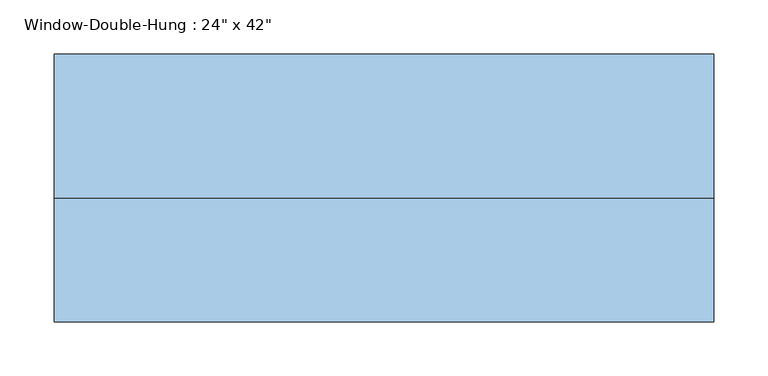
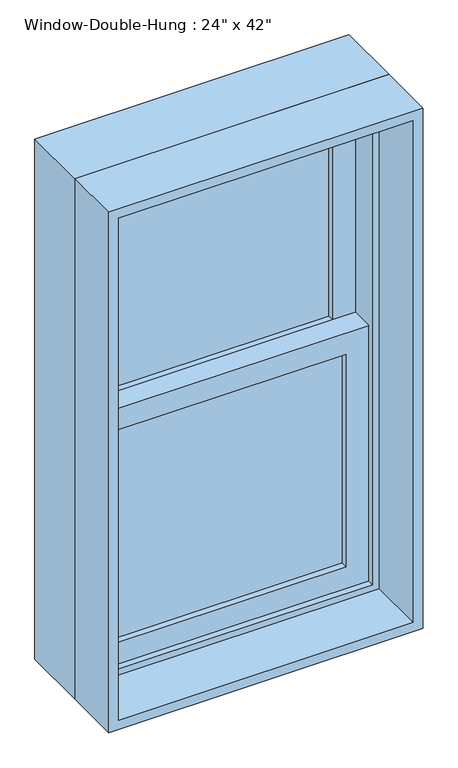
"""IFC4 building model written with IfcOpenShell, lengths in millimetres: window geometry."""

from ifc_helpers import new_model, si_unit, frame, origin, place, context, project, spatial, polyline, outline, extrude, source, transform, mapped, element, save


def window_d92165b9(model_context):
    return source(origin(), model_context, "Body", "SweptSolid", [
        extrude(outline(polyline([(228.6, 44.45), (228.6, 38.1), (-228.6, 38.1), (-228.6, 44.45), (228.6, 44.45)])), frame((0.0, 0.0, 990.6), z_axis=(0.0, 0.0, 1.0), x_axis=(1.0, 0.0, 0.0)), (0.0, 0.0, 1.0), 434.975),
        extrude(outline(polyline([(-228.6, 31.75), (228.6, 31.75), (228.6, 25.4), (-228.6, 25.4), (-228.6, 31.75)])), frame((0.0, 0.0, 990.6), z_axis=(0.0, 0.0, 1.0), x_axis=(1.0, 0.0, 0.0)), (0.0, 0.0, 1.0), 434.975),
        extrude(outline(polyline([(228.6, 88.9), (228.6, 82.55), (-228.6, 82.55), (-228.6, 88.9), (228.6, 88.9)])), frame((0.0, 0.0, 1470.025), z_axis=(0.0, 0.0, 1.0), x_axis=(1.0, 0.0, 0.0)), (0.0, 0.0, 1.0), 434.975),
        extrude(outline(polyline([(-228.6, 76.2), (228.6, 76.2), (228.6, 69.85), (-228.6, 69.85), (-228.6, 76.2)])), frame((0.0, 0.0, 1470.025), z_axis=(0.0, 0.0, 1.0), x_axis=(1.0, 0.0, 0.0)), (0.0, 0.0, 1.0), 434.975),
        extrude(outline(polyline([(1470.025, -273.05), (946.15, -273.05), (946.15, 273.05), (1470.025, 273.05), (1470.025, -273.05)]), holes=[polyline([(1425.575, 228.6), (990.6, 228.6), (990.6, -228.6), (1425.575, -228.6), (1425.575, 228.6)])]), frame((0.0, 12.7, 0.0), z_axis=(0.0, 1.0, 0.0), x_axis=(0.0, 0.0, 1.0)), (0.0, 0.0, 1.0), 44.45),
        extrude(outline(polyline([(1949.45, -273.05), (1425.575, -273.05), (1425.575, 273.05), (1949.45, 273.05), (1949.45, -273.05)]), holes=[polyline([(1905.0, 228.6), (1470.025, 228.6), (1470.025, -228.6), (1905.0, -228.6), (1905.0, 228.6)])]), frame((0.0, 57.15, 0.0), z_axis=(0.0, 1.0, 0.0), x_axis=(0.0, 0.0, 1.0)), (0.0, 0.0, 1.0), 44.45),
        extrude(outline(polyline([(1981.2, -304.8), (914.4, -304.8), (914.4, 304.8), (1981.2, 304.8), (1981.2, -304.8)]), holes=[polyline([(1949.45, 273.05), (946.15, 273.05), (946.15, -273.05), (1949.45, -273.05), (1949.45, 273.05)])]), frame((0.0, 0.0, 0.0), z_axis=(0.0, 1.0, 0.0), x_axis=(0.0, 0.0, 1.0)), (0.0, 0.0, 1.0), 133.35),
        extrude(outline(polyline([(1981.2, 304.8), (1981.2, -304.8), (914.4, -304.8), (914.4, 304.8), (1981.2, 304.8)]), holes=[polyline([(1962.15, 285.75), (933.45, 285.75), (933.45, -285.75), (1962.15, -285.75), (1962.15, 285.75)])]), frame((0.0, -114.3, 0.0), z_axis=(0.0, 1.0, 0.0), x_axis=(0.0, 0.0, 1.0)), (0.0, 0.0, 1.0), 114.3),
    ])


if __name__ == "__main__":
    model = new_model("IFC4")
    model_context = context("Model", 3, world=origin())
    ifc_project = project(units=[si_unit("LENGTHUNIT", "METRE", prefix="MILLI")], contexts=[model_context])
    site = spatial("IfcSite", under=ifc_project)
    building = spatial("IfcBuilding", under=site)
    placement = place(None, origin())
    window_shape = window_d92165b9(model_context)
    element("IfcWindow", 1, ObjectType="Window-Double-Hung : 24\" x 42\"", at=placement, inside=building, context=model_context, shape_type="MappedRepresentation", body=[
        mapped(window_shape, transform((0.0, 0.0, 0.0), x_axis=(1.0, 0.0, 0.0), y_axis=(0.0, 1.0, 0.0), z_axis=(0.0, 0.0, 1.0))),
    ])
    save(model, "model.ifc")

# Revit data of these elements
# Type "Window-Double-Hung : 24\" x 42\""
#   Type Mark = "10"
#   Fire Rating = "0.5h"
#   Construction Type Id = "DG-DR"
#   Assembly Code = "B2020100"
#   Analytic Construction = "Double glazing - domestic"
#   Wall Thickness [instance default] = 0' - 6"
#   Window Inset [instance default] = 0' - 0"
#   Visual Light Transmittance = 0.81
#   Thermal Resistance (R) = 1.8146 (h·ft²·°F)/BTU
#   Solar Heat Gain Coefficient = 0.76
#   Muntin Width = 1' - 6"
#   Muntin Height = 1' - 5 1/8"
#   Interior Wall Closure [instance default] = 0' - 1 1/2"
#   Rough Width = 2' - 0 1/2"
#   Rough Height = 3' - 6 1/2"
#   Frame Extension [instance default] = 0' - 1 1/4"
#   Exterior Wall Closure [instance default] = 0' - 0 1/2"
#   Extension Jamb [instance default] = 0' - 1 1/2"
#   Heat Transfer Coefficient (U) = 0.5511 BTU/(h·ft²·°F)
#   Height = 3' - 6"
#   Width = 2' - 0"
#   Define Thermal Properties by = 1
#   Top Muntin Visibility = yes
#   Indicator Visibility [instance default] = yes
#   Extension Jamb Visibility [instance default] = yes
#   Interior Trim Visibility [instance default] = yes
#   Exterior Trim Visibility [instance default] = yes
#   Define Thermal Properties by = 1
#   Bottom Muntin Visibility = yes
#   Muntin Pattern = Muntin Pattern_2x2 : Muntin Pattern_2x2
#   Interior Trim Material = Wood - Stained
#   Interior Trim = Trim-Window-Interior-Flat : Picture Frame
#   Exterior Trim Material = Clad - White
#   Exterior Trim = Trim-Window-Exterior-Flat : with Sill
#   Glass Panel Material = Glass
#   Exterior Frame Material = Clad - White
#   Interior Frame Material = Wood - Stained
#   Wall Closure = (empty or 0)
# Element 1 (IfcWindow, "Window-Double-Hung : 24\" x 42\"")
#   Wall Thickness = 0' - 9"
#   Extension Jamb = 0' - 4 1/2"
#   Materials on its faces: "Wood - Stained", "Glass", "Clad - White"
# Materials
#   "Wood - Stained": class "Wood", colour RGB 224 178 126, transparency 0, Cost = 0
#   "Clad - White": class "Wood", colour RGB 242 242 238, transparency 0, Cost = 0
#   "Glass": class "Glass", colour RGB 0 128 192, transparency 0.75, Description = "Soda Lime Glass", Cost = 0
